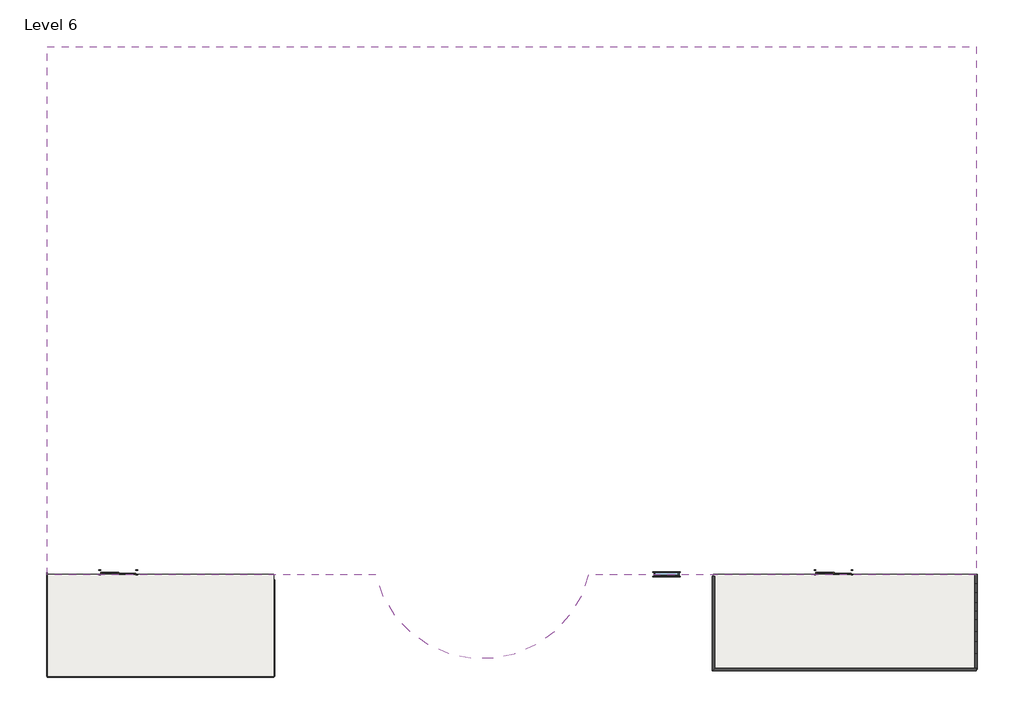
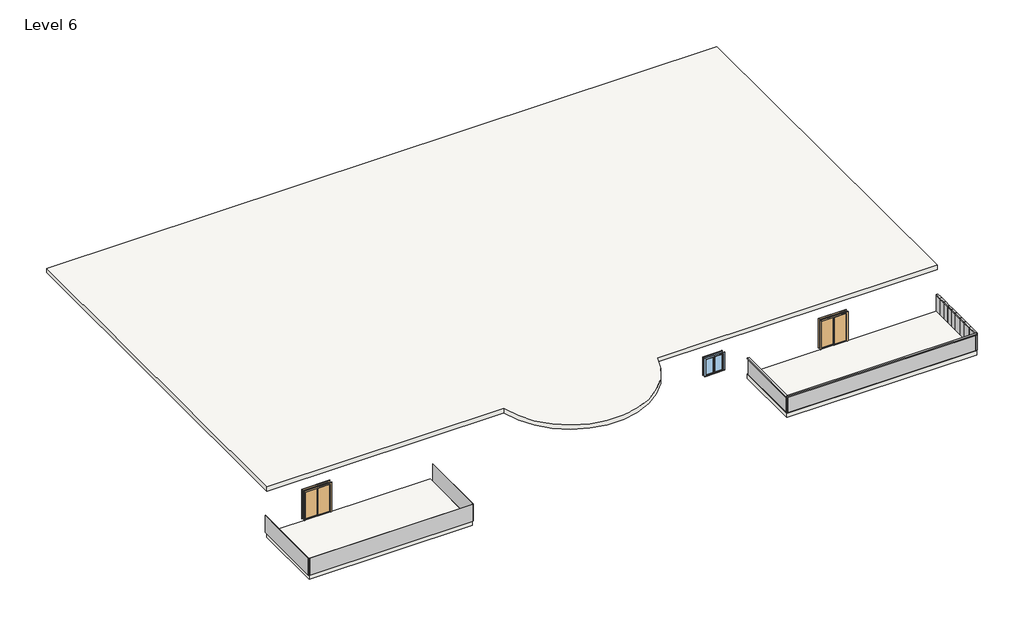
# One storey: 14 plates, 12 members, 3 slabs, 2 doors, 1 window.
"""IFC4 building model written with IfcOpenShell, lengths in millimetres."""

from ifc_helpers import new_model, si_unit, point, frame, frame_2d, origin, place, context, project, spatial, polyline, circle_curve, trimmed, segment, composite_curve, outline, extrude, transform, mapped, element, save
from components import door_076b30e0, member_75074519, member_47bfaf8a, member_7cfea1b5, member_15823cb3, member_2fb86761, member_69a911c1, member_b955a9e9, member_d7cde369, member_fc190105, system_panel_glazed_7b5ce646, system_panel_glazed_7af1c9c3, system_panel_glazed_f1530dac, system_panel_glazed_a18a7e0a, system_panel_glazed_7cd9bc56, system_panel_glazed_f69cdbc3, system_panel_glazed_d4b66054, system_panel_glazed_111ae4d9, system_panel_glazed_b96adab1, system_panel_glazed_2dfb9705, system_panel_glazed_974ae443, window_0862ab64

model = new_model("IFC4")

# Units and contexts
model_context = context("Model", 3, world=origin())
ifc_project = project(units=[si_unit("LENGTHUNIT", "METRE", prefix="MILLI")], contexts=[model_context])

# Site, building, storey
site = spatial("IfcSite", under=ifc_project)
building = spatial("IfcBuilding", under=site)
storey = spatial("IfcBuildingStorey", under=building, Name="Level 6", Elevation=9753.6)

# Doors
placement = place(None, origin())
door_shape = door_076b30e0(model_context)
element("IfcDoor", 1, ObjectType="Door-Double-Sliding : 68\" x 80\"", at=placement, inside=storey, context=model_context, shape_type="MappedRepresentation", body=[
    mapped(door_shape, transform((-16369.385279, -12227.7237084, 9753.6), x_axis=(-1.0, 0.0, 0.0), y_axis=(0.0, -1.0, 0.0), z_axis=(0.0, 0.0, 1.0))),
])
element("IfcDoor", 2, ObjectType="Door-Double-Sliding : 68\" x 80\"", at=placement, inside=storey, context=model_context, shape_type="MappedRepresentation", body=[
    mapped(door_shape, transform((18530.214721, -12227.7237084, 9753.6), x_axis=(-1.0, 0.0, 0.0), y_axis=(0.0, -1.0, 0.0), z_axis=(0.0, 0.0, 1.0))),
])

# Members
member_shape = member_75074519(model_context)
element("IfcMember", 3, ObjectType="Rectangular Mullion : 2.5\" x 5\" rectangular", at=placement, inside=storey, context=model_context, shape_type="MappedRepresentation", body=[
    mapped(member_shape, transform((25489.814721, -17089.2030397, 10972.8), x_axis=(0.0, -1.0, 0.0), y_axis=(1.0, 0.0, 0.0), z_axis=(0.0, 0.0, 1.0))),
])
member_2_shape = member_47bfaf8a(model_context)
element("IfcMember", 4, ObjectType="Rectangular Mullion : 2.5\" x 5\" rectangular", at=placement, inside=storey, context=model_context, shape_type="MappedRepresentation", body=[
    mapped(member_2_shape, transform((25489.814721, -14650.8030397, 10972.8), x_axis=(0.0, 0.0, 1.0), y_axis=(1.0, 0.0, 0.0), z_axis=(0.0, 1.0, 0.0))),
])
element("IfcMember", 5, ObjectType="Rectangular Mullion : 2.5\" x 5\" rectangular", at=placement, inside=storey, context=model_context, shape_type="MappedRepresentation", body=[
    mapped(member_2_shape, transform((25489.814721, -15717.6030397, 10972.8), x_axis=(0.0, 0.0, 1.0), y_axis=(1.0, 0.0, 0.0), z_axis=(0.0, 1.0, 0.0))),
])
member_3_shape = member_7cfea1b5(model_context)
element("IfcMember", 6, ObjectType="Rectangular Mullion : 2.5\" x 5\" rectangular", at=placement, inside=storey, context=model_context, shape_type="MappedRepresentation", body=[
    mapped(member_3_shape, transform((25489.814721, -14244.4030397, 10972.8), x_axis=(0.0, 0.0, 1.0), y_axis=(1.0, 0.0, 0.0), z_axis=(0.0, 1.0, 0.0))),
])
member_4_shape = member_15823cb3(model_context)
element("IfcMember", 7, ObjectType="Rectangular Mullion : 2.5\" x 5\" rectangular", at=placement, inside=storey, context=model_context, shape_type="MappedRepresentation", body=[
    mapped(member_4_shape, transform((25489.814721, -15260.4030397, 10972.8), x_axis=(0.0, 0.0, 1.0), y_axis=(1.0, 0.0, 0.0), z_axis=(0.0, 1.0, 0.0))),
])
member_5_shape = member_2fb86761(model_context)
element("IfcMember", 8, ObjectType="Rectangular Mullion : 2.5\" x 5\" rectangular", at=placement, inside=storey, context=model_context, shape_type="MappedRepresentation", body=[
    mapped(member_5_shape, transform((25489.814721, -12908.4168188, 10972.8), x_axis=(0.0, 0.0, 1.0), y_axis=(1.0, 0.0, 0.0), z_axis=(0.0, 1.0, 0.0))),
])
element("IfcMember", 9, ObjectType="Rectangular Mullion : 2.5\" x 5\" rectangular", at=placement, inside=storey, context=model_context, shape_type="MappedRepresentation", body=[
    mapped(member_5_shape, transform((25489.814721, -13360.5099293, 10972.8), x_axis=(0.0, 0.0, 1.0), y_axis=(1.0, 0.0, 0.0), z_axis=(0.0, 1.0, 0.0))),
])
member_6_shape = member_69a911c1(model_context)
element("IfcMember", 10, ObjectType="Rectangular Mullion : 2.5\" x 5\" rectangular", at=placement, inside=storey, context=model_context, shape_type="MappedRepresentation", body=[
    mapped(member_6_shape, transform((25489.814721, -13812.6030397, 10972.8), x_axis=(0.0, 0.0, 1.0), y_axis=(1.0, 0.0, 0.0), z_axis=(0.0, 1.0, 0.0))),
])
member_7_shape = member_b955a9e9(model_context)
element("IfcMember", 11, ObjectType="Rectangular Mullion : 2.5\" x 5\" rectangular", at=placement, inside=storey, context=model_context, shape_type="MappedRepresentation", body=[
    mapped(member_7_shape, transform((25489.814721, -16327.2030397, 10972.8), x_axis=(0.0, 0.0, 1.0), y_axis=(1.0, 0.0, 0.0), z_axis=(0.0, 1.0, 0.0))),
])
element("IfcMember", 12, ObjectType="Rectangular Mullion : 2.5\" x 5\" rectangular", at=placement, inside=storey, context=model_context, shape_type="MappedRepresentation", body=[
    mapped(member_5_shape, transform((25489.814721, -12456.3237084, 10972.8), x_axis=(0.0, 0.0, 1.0), y_axis=(1.0, 0.0, 0.0), z_axis=(0.0, 1.0, 0.0))),
])
member_8_shape = member_d7cde369(model_context)
element("IfcMember", 13, ObjectType="Rectangular Mullion : 2.5\" x 5\" rectangular", at=placement, inside=storey, context=model_context, shape_type="MappedRepresentation", body=[
    mapped(member_8_shape, transform((12667.5594464, -17089.2030397, 10972.8), x_axis=(0.0, 0.0, 1.0), y_axis=(-1.0, 0.0, 0.0), z_axis=(0.0, -1.0, 0.0))),
])
member_9_shape = member_fc190105(model_context)
element("IfcMember", 14, ObjectType="Rectangular Mullion : 2.5\" x 5\" rectangular", at=placement, inside=storey, context=model_context, shape_type="MappedRepresentation", body=[
    mapped(member_9_shape, transform((25489.814721, -17089.2030397, 10972.8), x_axis=(0.0, 0.0, 1.0), y_axis=(0.0, -1.0, 0.0), z_axis=(1.0, 0.0, 0.0))),
])

# Plates
system_panel_glazed_shape = system_panel_glazed_7b5ce646(model_context)
element("IfcPlate", 15, ObjectType="System Panel : Glazed", at=placement, inside=storey, context=model_context, shape_type="MappedRepresentation", body=[
    mapped(system_panel_glazed_shape, transform((25489.814721, -16676.4530397, 9753.6), x_axis=(0.0, 1.0, 0.0), y_axis=(-1.0, 0.0, 0.0), z_axis=(0.0, 0.0, 1.0))),
])
system_panel_glazed_2_shape = system_panel_glazed_7af1c9c3(model_context)
element("IfcPlate", 16, ObjectType="System Panel : Glazed", at=placement, inside=storey, context=model_context, shape_type="MappedRepresentation", body=[
    mapped(system_panel_glazed_2_shape, transform((25489.814721, -16022.4030397, 9753.6), x_axis=(0.0, 1.0, 0.0), y_axis=(-1.0, 0.0, 0.0), z_axis=(0.0, 0.0, 1.0))),
])
element("IfcPlate", 17, ObjectType="System Panel : Glazed", at=placement, inside=storey, context=model_context, shape_type="MappedRepresentation", body=[
    mapped(system_panel_glazed_2_shape, transform((25489.814721, -14955.6030397, 9753.6), x_axis=(0.0, 1.0, 0.0), y_axis=(-1.0, 0.0, 0.0), z_axis=(0.0, 0.0, 1.0))),
])
system_panel_glazed_3_shape = system_panel_glazed_f1530dac(model_context)
element("IfcPlate", 18, ObjectType="System Panel : Glazed", at=placement, inside=storey, context=model_context, shape_type="MappedRepresentation", body=[
    mapped(system_panel_glazed_3_shape, transform((25489.814721, -14447.6030397, 9753.6), x_axis=(0.0, 1.0, 0.0), y_axis=(-1.0, 0.0, 0.0), z_axis=(0.0, 0.0, 1.0))),
])
system_panel_glazed_4_shape = system_panel_glazed_a18a7e0a(model_context)
element("IfcPlate", 19, ObjectType="System Panel : Glazed", at=placement, inside=storey, context=model_context, shape_type="MappedRepresentation", body=[
    mapped(system_panel_glazed_4_shape, transform((25489.814721, -15489.0030397, 9753.6), x_axis=(0.0, 1.0, 0.0), y_axis=(-1.0, 0.0, 0.0), z_axis=(0.0, 0.0, 1.0))),
])
system_panel_glazed_5_shape = system_panel_glazed_7cd9bc56(model_context)
element("IfcPlate", 20, ObjectType="System Panel : Glazed", at=placement, inside=storey, context=model_context, shape_type="MappedRepresentation", body=[
    mapped(system_panel_glazed_5_shape, transform((19078.6870837, -17089.2030397, 9753.6), x_axis=(1.0, 0.0, 0.0), y_axis=(0.0, 1.0, 0.0), z_axis=(0.0, 0.0, 1.0))),
])
system_panel_glazed_6_shape = system_panel_glazed_f69cdbc3(model_context)
element("IfcPlate", 21, ObjectType="System Panel : Glazed", at=placement, inside=storey, context=model_context, shape_type="MappedRepresentation", body=[
    mapped(system_panel_glazed_6_shape, transform((25489.814721, -14028.5030397, 9753.6), x_axis=(0.0, 1.0, 0.0), y_axis=(-1.0, 0.0, 0.0), z_axis=(0.0, 0.0, 1.0))),
])
system_panel_glazed_7_shape = system_panel_glazed_d4b66054(model_context)
element("IfcPlate", 22, ObjectType="System Panel : Glazed", at=placement, inside=storey, context=model_context, shape_type="MappedRepresentation", body=[
    mapped(system_panel_glazed_7_shape, transform((25489.814721, -13586.5564845, 9753.6), x_axis=(0.0, 1.0, 0.0), y_axis=(-1.0, 0.0, 0.0), z_axis=(0.0, 0.0, 1.0))),
])
element("IfcPlate", 23, ObjectType="System Panel : Glazed", at=placement, inside=storey, context=model_context, shape_type="MappedRepresentation", body=[
    mapped(system_panel_glazed_7_shape, transform((25489.814721, -13134.4633741, 9753.6), x_axis=(0.0, 1.0, 0.0), y_axis=(-1.0, 0.0, 0.0), z_axis=(0.0, 0.0, 1.0))),
])
element("IfcPlate", 24, ObjectType="System Panel : Glazed", at=placement, inside=storey, context=model_context, shape_type="MappedRepresentation", body=[
    mapped(system_panel_glazed_7_shape, transform((25489.814721, -12682.3702636, 9753.6), x_axis=(0.0, 1.0, 0.0), y_axis=(-1.0, 0.0, 0.0), z_axis=(0.0, 0.0, 1.0))),
])
system_panel_glazed_8_shape = system_panel_glazed_111ae4d9(model_context)
element("IfcPlate", 25, ObjectType="System Panel : Glazed", at=placement, inside=storey, context=model_context, shape_type="MappedRepresentation", body=[
    mapped(system_panel_glazed_8_shape, transform((12667.5594464, -14823.5633741, 9753.6), x_axis=(0.0, -1.0, 0.0), y_axis=(1.0, 0.0, 0.0), z_axis=(0.0, 0.0, 1.0))),
])
system_panel_glazed_9_shape = system_panel_glazed_b96adab1(model_context)
element("IfcPlate", 26, ObjectType="System Panel : Glazed", at=placement, inside=storey, context=model_context, shape_type="MappedRepresentation", body=[
    mapped(system_panel_glazed_9_shape, transform((-14302.7926538, -17427.8940509, 9753.6), x_axis=(-1.0, 0.0, 0.0), y_axis=(0.0, -1.0, 0.0), z_axis=(0.0, 0.0, 1.0))),
])
system_panel_glazed_10_shape = system_panel_glazed_2dfb9705(model_context)
element("IfcPlate", 27, ObjectType="System Panel : Glazed", at=placement, inside=storey, context=model_context, shape_type="MappedRepresentation", body=[
    mapped(system_panel_glazed_10_shape, transform((-19823.785279, -14891.3088796, 9753.6), x_axis=(0.0, 1.0, 0.0), y_axis=(-1.0, 0.0, 0.0), z_axis=(0.0, 0.0, 1.0))),
])
system_panel_glazed_11_shape = system_panel_glazed_974ae443(model_context)
element("IfcPlate", 28, ObjectType="System Panel : Glazed", at=placement, inside=storey, context=model_context, shape_type="MappedRepresentation", body=[
    mapped(system_panel_glazed_11_shape, transform((-8781.8000285, -15073.3473909, 9753.6), x_axis=(0.0, -1.0, 0.0), y_axis=(1.0, 0.0, 0.0), z_axis=(0.0, 0.0, 1.0))),
])

# Slabs
element("IfcSlab", 29, ObjectType="Generic - 12\"", at=placement, inside=storey, context=model_context, shape_type="SweptSolid", body=[
    extrude(outline(composite_curve([segment(polyline([(25489.814721, 13322.6839017), (25489.814721, -12483.7160983), (6571.5594464, -12483.7160983)]), True, "CONTINUOUS"), segment(trimmed(circle_curve(frame_2d((1385.214721, -11253.083057)), 5330.3498284), [point((6571.5594464, -12483.7160983))], [point((-3801.1300045, -12483.7160983))], False, "CARTESIAN"), True, "CONTINUOUS"), segment(polyline([(-3801.1300045, -12483.7160983), (-19823.785279, -12483.7160983), (-19823.785279, 13322.6839017), (25489.814721, 13322.6839017)]), True, "CONTINUOUS")], self_intersect=False)), frame((0.0, 0.0, 12750.6634343), z_axis=(0.0, 0.0, 1.0), x_axis=(1.0, 0.0, 0.0)), (0.0, 0.0, 1.0), 304.8),
])
element("IfcSlab", 30, ObjectType="Generic - 12\"", at=placement, inside=storey, context=model_context, shape_type="SweptSolid", body=[
    extrude(outline(polyline([(25489.814721, -12456.3237084), (25489.814721, -17089.2030397), (12667.5594464, -17089.2030397), (12667.5594464, -12456.3237084), (25489.814721, -12456.3237084)])), frame((0.0, 0.0, 9448.8), z_axis=(0.0, 0.0, 1.0), x_axis=(1.0, 0.0, 0.0)), (0.0, 0.0, 1.0), 304.8),
])
element("IfcSlab", 31, ObjectType="Generic - 12\"", at=placement, inside=storey, context=model_context, shape_type="SweptSolid", body=[
    extrude(outline(polyline([(-8781.8000285, -12456.3237084), (-8781.8000285, -17427.8940509), (-19823.785279, -17427.8940509), (-19823.785279, -12456.3237084), (-8781.8000285, -12456.3237084)])), frame((0.0, 0.0, 9448.8), z_axis=(0.0, 0.0, 1.0), x_axis=(1.0, 0.0, 0.0)), (0.0, 0.0, 1.0), 304.8),
])

# Window
window_shape = window_0862ab64(model_context)
element("IfcWindow", 32, ObjectType="Casement Dbl with Trim : 48\" x 48\"", at=placement, inside=storey, context=model_context, shape_type="MappedRepresentation", body=[
    mapped(window_shape, transform((10381.5594464, -12437.2737084, 9753.6), x_axis=(-1.0, 0.0, 0.0), y_axis=(0.0, -1.0, 0.0), z_axis=(0.0, 0.0, 1.0))),
])

save(model, "model.ifc")

# Revit data of these elements
# Type "Door-Double-Sliding : 68\" x 80\""
#   Type Mark = "10"
#   Construction Type Id = "opn-d45"
#   Assembly Code = "C1020"
#   Analytic Construction = "Wood frame, double glass door "
#   Thickness = 0' - 2"
#   Thermal Resistance (R) = 1.8150 (h·ft²·°F)/BTU
#   Heat Transfer Coefficient (U) = 0.5510 BTU/(h·ft²·°F)
#   Height = 6' - 8"
#   Rail Width = 0' - 2"
#   Stiles = 0' - 2"
#   Trim Projection Ext = 0' - 1"
#   Trim Projection Int = 0' - 1"
#   Trim Width = 0' - 3"
#   Width = 5' - 8"
#   Define Thermal Properties by = 1
#   Glazing = Glass
#   Panel Material = Wood - Birch - Solid Stained Light Low Gloss
#   Trim Material = Paint - Sienna
#   Visual Light Transmittance = 0
#   Solar Heat Gain Coefficient = 0
#   Function = (empty or 0)
#   Wall Closure = (empty or 0)
# Type "Rectangular Mullion : 2.5\" x 5\" rectangular"
#   built-in parameter 1007304 = 0.416667 (stored number, unit not read)
#   built-in parameter 1007301 = 0.104167 (stored number, unit not read)
#   built-in parameter 1007300 = 0.104167 (stored number, unit not read)
# Type "System Panel : Glazed"
#   Construction Type Id = "GSP4R"
#   Analytic Construction = "1/8 in Pilkington single glazing"
#   Visual Light Transmittance = 0.9
#   Solar Heat Gain Coefficient = 0.86
#   Heat Transfer Coefficient (U) = 1.18115 BTU/(h·ft²·°F)
# Type "Generic - 12\""
#   Assembly Code = "B1010"
#   Function = 0
#   Layers, outside or top first: 1' - 0" no material (function 1)
# Type "Casement Dbl with Trim : 48\" x 48\""
#   Type Mark = "34"
#   Construction Type Id = "GSP4R"
#   Assembly Code = "B2020100"
#   Analytic Construction = "1/8 in Pilkington single glazing"
#   Visual Light Transmittance = 0.9
#   Solar Heat Gain Coefficient = 0.78
#   Heat Transfer Coefficient (U) = 0.6496 BTU/(h·ft²·°F)
#   Height = 4' - 0"
#   Default Sill Height = 3' - 0"
#   Trim Projection - Ext. = 0' - 0 1/2"
#   Trim Projection - Int. = 0' - 0 3/4"
#   Trim Width - Exterior = 0' - 3 1/2"
#   Trim Width - Interior = 0' - 3 1/2"
#   Width = 4' - 0"
#   Window Inset = 0' - 0 3/4"
#   Define Thermal Properties by = 1
#   Glass Pane Material = Glass
#   Sash Material = Sash
#   Trim Exterior Material = Trim
#   Trim Interior Material = Trim
#   Wall Closure = (empty or 0)
# Elements 1, 2 (IfcDoor, "Door-Double-Sliding : 68\" x 80\"")
#   Phase Created = New Construction
#   Materials on its faces: "Paint - Sienna", "Wood - Birch - Solid Stained Light Low Gloss", "Glass"
# Elements 3, 4, 5, 6, 7, 8, 9, 10, 11, 12, 13, 14 (IfcMember, "Rectangular Mullion : 2.5\" x 5\" rectangular")
#   Phase Created = New Construction
#   Materials on its faces: "Aluminum"
# Elements 15, 16, 17, 18, 19, 20, 21, 22, 23, 24, 25, 26, 27, 28 (IfcPlate, "System Panel : Glazed")
#   Phase Created = New Construction
#   Materials on its faces: "Glass"
# Element 29 (IfcSlab, "Generic - 12\"")
#   Height Offset From Level = 10' - 9.99462"
#   Phase Created = New Construction
#   Materials on its faces: "Default Floor"
# Elements 30, 31 (IfcSlab, "Generic - 12\"")
#   Height Offset From Level = 0' - 0"
#   Phase Created = New Construction
#   Materials on its faces: "Default Floor"
# Element 32 (IfcWindow, "Casement Dbl with Trim : 48\" x 48\"")
#   Mark = "14"
#   Phase Created = New Construction
#   Materials on its faces: "Sash", "Trim", "Glass"
# Materials
#   "Glass": class "Glass", colour RGB 0 128 192, transparency 0.75, Description = "Soda Lime Glass", Cost = 0
#   "Wood - Birch - Solid Stained Light Low Gloss": class "Wood", colour RGB 210 159 95, transparency 0, Cost = 0
#   "Paint - Sienna": colour RGB 118 70 51, transparency 0, Cost = 0
#   "Sash": class "Wood", colour RGB 224 178 126, transparency 0
#   "Trim": class "Wood", colour RGB 224 178 126, transparency 0
#   "Aluminum": class "Metal", colour RGB 247 247 247, transparency 0, Description = "Aluminum 6061", Cost = 0
#   "Default Floor": colour RGB 128 128 128, transparency 0
